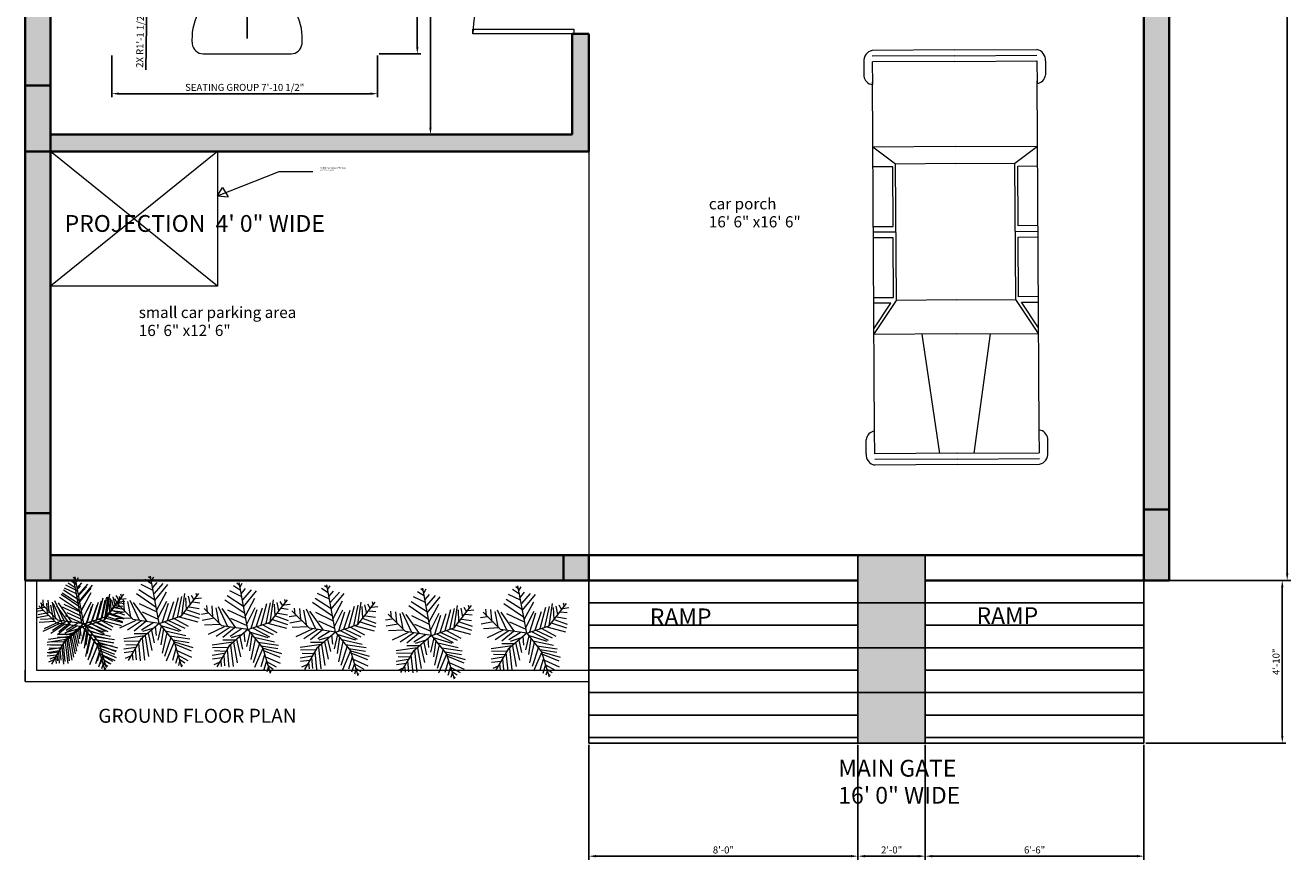
# Model space of a CAD drawing. Units: inches. Extents: x 2369 to 4208, y 1650 to 4492.
# Tile 1 of 6: x 2369 to 2820, y 1650 to 1948. Entities that reach past the tile are written whole.
import ezdxf

# ---------------------------------------------------------------- set-up
doc = ezdxf.new("R2010")
doc.units = ezdxf.units.IN
for name, color, linetype, lineweight in [('A-ANNO-DIMS', 2, 'Continuous', 13), ('A-ANNO-TEXT', 7, 'Continuous', 18), ('A-AREA-IDEN', 7, 'Continuous', 18), ('A-COLS', 7, 'Continuous', 35), ('A-COLS-PATT', 7, 'Continuous', 13), ('A-DOOR', 4, 'Continuous', 18), ('A-FLOR-PARK', 7, 'Continuous', 18), ('A-FLOR-RAMP', 7, 'Continuous', 25), ('A-FLOR-RAMP-PATT', 252, 'Continuous', 13), ('A-FURN', 8, 'Continuous', 18), ('A-FURN-VEHI', 8, 'Continuous', 13), ('A-WALL', 7, 'Continuous', 35), ('A-WALL-PATT', 252, 'Continuous', 13), ('L-PLNT-BEDS', 3, 'Continuous', 18), ('L-PLNT-TREE', 3, 'Continuous', 13), ('P-EQPM-TANK', 7, 'Continuous', 18)]:
    doc.layers.add(name, color=color, linetype=linetype, lineweight=lineweight)
doc.styles.get("Standard").update_dxf_attribs({"font": 'arial.ttf'})
doc.dimstyles.new('Copy of ISO-25', dxfattribs={"dimtxt": 2.5, "dimasz": 2.5, "dimexe": 1.25, "dimexo": 0.625, "dimtad": 1, "dimdec": 1, "dimlunit": 4, "dimtxsty": 'Standard', "dimcen": 2.5, "dimadec": 0, "dimazin": 0, "dimtfac": 1, "dimtdec": 1, "dimtmove": 0, "dimatfit": 3, "dimfxl": 1, "dimarcsym": 0})

# ---------------------------------------------------------------- blocks, each defined once
blk = doc.blocks.new('*U4')
for p, q in [((-40, 0), (-40, 6)), ((0, 0), (0, 6))]:
    blk.add_line(p, q)
blk.add_lwpolyline([(0, 0), (0, -40), (-1.75, -40), (-1.75, 0)], close=True)
blk.add_arc((0, 0), 40, 180, 270)
blk = doc.blocks.new('*D8')
at = {"layer": 'A-ANNO-DIMS', "color": 0, "lineweight": -2, "transparency": 16777216}
for p, q in [((2777.53, 2469.98), (2820.25, 2469.98)), ((2819, 2467.48), (2819, 1752.48)), ((2777.53, 1749.98), (2820.25, 1749.98))]:
    blk.add_line(p, q, dxfattribs=at)
at = {"layer": 'A-ANNO-DIMS', "color": 0, "transparency": 16777216}
for points in [[(2818.58, 2467.48), (2819.41, 2467.48), (2819, 2469.98)], [(2818.58, 1752.48), (2819.41, 1752.48), (2819, 1749.98)]]:
    blk.add_solid(points, dxfattribs=at)
at = {"layer": 'Defpoints', "color": 0, "transparency": 16777216}
for p in [(2776.9, 2469.98), (2776.9, 1749.98), (2819, 1749.98)]:
    blk.add_point(p, dxfattribs=at)
at = {"layer": 'A-ANNO-DIMS', "color": 0, "transparency": 16777216, "insert": (2817.1, 2109.98), "char_height": 2.5, "attachment_point": 5, "rotation": 90}
blk.add_mtext("60'", dxfattribs=at)
blk = doc.blocks.new('*D30')
at = {"layer": 'A-ANNO-DIMS', "color": 0, "lineweight": -2, "transparency": 16777216}
for p, q in [((2563.28, 2052.98), (2512.16, 2052.98)), ((2513.41, 2050.48), (2513.41, 1911.48)), ((2563.28, 1908.98), (2512.16, 1908.98))]:
    blk.add_line(p, q, dxfattribs=at)
at = {"layer": 'A-ANNO-DIMS', "color": 0, "transparency": 16777216}
for points in [[(2512.99, 2050.48), (2513.82, 2050.48), (2513.41, 2052.98)], [(2512.99, 1911.48), (2513.82, 1911.48), (2513.41, 1908.98)]]:
    blk.add_solid(points, dxfattribs=at)
at = {"layer": 'Defpoints', "color": 0, "transparency": 16777216}
for p in [(2563.9, 2052.98), (2513.41, 1908.98), (2563.9, 1908.98)]:
    blk.add_point(p, dxfattribs=at)
at = {"layer": 'A-ANNO-DIMS', "color": 0, "transparency": 16777216, "insert": (2511.53, 1980.98), "char_height": 2.5, "attachment_point": 5, "rotation": 90}
blk.add_mtext("12'", dxfattribs=at)
blk = doc.blocks.new('*U34')
for p, q in [((-7.288, 39.707), (-21.778, 46.673)), ((-8.737, 47.138), (-17.069, 52.711)), ((-10.186, 53.64), (-13.084, 55.962)), ((0, 0), (-10.5, 57)), ((-9.099, 51.782), (-6.563, 55.962)), ((-7.65, 43.423), (-2.578, 49.46)), ((-5.839, 35.992), (4.667, 48.067)), ((-5.114, 27.632), (10.463, 46.673)), ((-3.665, 19.273), (-27.574, 35.527)), ((-5.114, 28.097), (-24.676, 40.636)), ((-2.941, 16.486), (8.652, 37.85)), ((16.259, 5.805), (23.142, 31.348)), ((22.055, 7.198), (27.489, 32.277)), ((27, 9), (48, 36)), ((27.127, 9.056), (31.112, 35.992)), ((31.836, 30.883), (32.561, 16.486)), ((35.096, 32.741), (37.27, 22.524)), ((38.719, 34.134), (41.979, 28.561)), ((43.791, 29.954), (51.036, 30.883)), ((44.153, 36.456), (45.239, 32.741)), ((-47.498, 19.737), (-55.83, 18.344)), ((-31.5, 4.5), (-52.5, 25.5)), ((-48.585, 21.131), (-49.309, 29.026)), ((-43.513, 28.561), (-42.427, 15.558)), ((-38.442, 26.239), (-34.819, 7.663)), ((-35.544, 28.097), (-24.314, 3.947)), ((-14.533, 2.09), (-30.834, 25.31)), ((-24.314, 23.917), (-2.941, 13.7)), ((-1.129, 6.734), (9.014, 26.704)), ((3.942, 1.625), (11.187, 24.381)), ((10.101, 3.483), (17.708, 26.239)), ((33.285, 16.486), (48.862, 10.913)), ((36.183, 19.737), (48.137, 17.88)), ((40.53, 25.775), (48.862, 24.846)), ((-40.615, 13.7), (-55.105, 10.913)), ((-33.37, 6.269), (-52.207, 5.34)), ((-28.299, 3.483), (-47.86, -5.805)), ((-21.416, 3.018), (-38.079, -8.128)), ((0, 0), (-31.5, 4.5)), ((-15.982, 2.09), (-30.11, -9.521)), ((0, 0), (-22.5, -19.5)), ((-6.563, 1.161), (-21.416, -8.128)), ((-20.691, 13.7), (-1.129, 4.876)), ((0, 0), (27, 9)), ((0, 0), (18, -22.5)), ((6.478, 1.625), (26.04, -8.592)), ((11.187, 3.483), (30.749, -5.805)), ((18.07, 5.805), (35.096, -3.483)), ((24.229, 7.663), (46.688, 1.625)), ((29.662, 12.307), (48.137, 6.269)), ((-17.431, -15.094), (-42.789, -18.809)), ((-15.257, -12.772), (-30.11, -12.772)), ((-6.563, -5.805), (-19.967, -9.985)), ((-17.069, -15.094), (-12.721, -40.172)), ((-13.446, -11.378), (-8.737, -32.741)), ((-9.461, -8.592), (-6.201, -23.453)), ((-4.752, -3.483), (-3.665, -14.629)), ((2.493, -3.019), (-1.491, -20.202)), ((1.769, -2.555), (24.229, -9.521)), ((5.029, -6.27), (2.131, -25.775)), ((9.014, -11.378), (3.58, -35.992)), ((7.565, -9.056), (32.198, -14.629)), ((12.274, -15.094), (36.907, -18.809)), ((-28.299, -29.026), (-42.789, -31.348)), ((-24.314, -21.596), (-42.427, -22.06)), ((-26.849, -26.24), (-40.253, -25.775)), ((-22.5, -19.5), (-37.5, -45)), ((-25.038, -23.918), (-22.865, -45.281)), ((-20.691, -18.345), (-17.793, -44.352)), ((14.085, -16.951), (6.478, -40.172)), ((18.07, -22.524), (8.289, -45.745)), ((20.244, -30.419), (15.897, -44.816)), ((16.259, -19.738), (36.183, -22.989)), ((18, -22.5), (27, -52.5)), ((18.433, -22.524), (40.53, -29.026)), ((19.157, -25.311), (38.719, -33.206)), ((-30.834, -34.135), (-42.427, -35.528)), ((-34.457, -39.708), (-40.978, -42.494)), ((-32.646, -36.921), (-31.921, -44.352)), ((-29.023, -30.884), (-27.936, -43.887)), ((22.78, -37.85), (19.519, -48.532)), ((21.331, -32.741), (39.081, -40.636)), ((22.78, -38.314), (34.372, -44.816)), ((24.591, -45.745), (23.142, -50.854)), ((24.591, -43.423), (30.749, -47.603)), ((26.764, -49.925), (28.213, -50.854))]:
    blk.add_line(p, q)
blk = doc.blocks.new('*U36')
for p, q in [((138, 1075), (308, 1075)), ((4818, 1075), (4649, 1075)), ((3, -10), (3, 974)), ((70, -10), (70, 973)), ((138, 973), (410, 973)), ((138, -10), (138, 971)), ((410, 973), (4581, 973)), ((1563, -10), (1563, 973)), ((1563, 973), (1969, 702)), ((1630, 973), (1936, 769)), ((1936, 769), (1936, 973)), ((2003, 973), (2003, 736)), ((2716, 736), (2716, 973)), ((2783, 702), (2783, 973)), ((2851, 973), (2851, 736)), ((3563, 736), (3563, 973)), ((3597, 702), (3801, 973)), ((3801, -10), (3801, 973)), ((4818, 973), (4547, 973)), ((4818, -10), (4818, 971)), ((4886, -10), (4886, 973)), ((4954, -10), (4954, 974)), ((1969, 702), (3597, 702)), ((1969, -10), (1969, 702)), ((2003, 736), (2716, 736)), ((2851, 736), (3563, 736)), ((3597, -10), (3597, 702)), ((138, 193), (1563, 396)), ((3, -11), (3, -995)), ((70, -10), (70, -994)), ((138, -11), (138, -992)), ((1563, -10), (1563, -994)), ((1969, -10), (1969, -723)), ((3597, -10), (3597, -723)), ((3801, -10), (3801, -994)), ((4818, -11), (4818, -992)), ((4886, -10), (4886, -994)), ((4954, -11), (4954, -995)), ((138, -214), (1563, -417)), ((1563, -994), (1969, -723)), ((1969, -723), (3597, -723)), ((2783, -723), (2783, -994)), ((3597, -723), (3801, -994)), ((1630, -994), (1936, -790)), ((1936, -790), (1936, -994)), ((2003, -994), (2003, -757)), ((2003, -757), (2716, -757)), ((2716, -757), (2716, -994)), ((2851, -757), (3563, -757)), ((2851, -994), (2851, -757)), ((3563, -757), (3563, -994)), ((138, -994), (410, -994)), ((410, -994), (4581, -994)), ((4818, -994), (4547, -994)), ((138, -1096), (308, -1096)), ((4818, -1096), (4649, -1096))]:
    blk.add_line(p, q)
for centre, radius, start, end in [((128, 946), 129, 85.6455, 168.0943), ((291, 956), 120, 8.1301, 81.87), ((4665, 956), 120, 98.13, 171.8699), ((4828, 946), 129, 11.9057, 94.3545), ((128, -967), 129, 191.9057, 274.3545), ((291, -977), 120, 278.13, 351.8699), ((4665, -977), 120, 188.1301, 261.87), ((4828, -967), 129, 265.6455, 348.0943)]:
    blk.add_arc(centre, radius, start, end)
blk = doc.blocks.new('A$C22FC404C')
for p, q in [((1200, 1302), (1200, 1942)), ((809, 1143), (363, 1602)), ((1594, 1139), (2045, 1594)), ((0, 760), (640, 751)), ((2400, 731), (1760, 735)), ((827, 0), (1623, 0))]:
    blk.add_line(p, q)
for centre, radius, start, end in [((1200, 742), 1200, 359.499, 179.1174), ((1200, 742), 1040, 359.4096, 179.1174), ((1200, 742), 560, 359.3286, 179.1174), ((323, 870), 341, 199.1309, 339.1039), ((2082, 839), 341, 200.8961, 340.8691), ((1225, 139), 500, 354.3583, 185.6417), ((827, 100), 100, 185.6417, 270), ((1623, 100), 100, 270, 354.3583)]:
    blk.add_arc(centre, radius, start, end)
blk = doc.blocks.new('*D55')
at = {"layer": 'A-ANNO-DIMS', "color": 0, "lineweight": -2, "transparency": 16777216}
for p, q in [((2399.8, 1937.17), (2399.8, 1922.34)), ((2494.51, 1937.17), (2494.51, 1922.34)), ((2402.3, 1923.59), (2492.01, 1923.59))]:
    blk.add_line(p, q, dxfattribs=at)
at = {"layer": 'A-ANNO-DIMS', "color": 0, "transparency": 16777216}
for points in [[(2402.3, 1924.01), (2402.3, 1923.18), (2399.8, 1923.59)], [(2492.01, 1924.01), (2492.01, 1923.18), (2494.51, 1923.59)]]:
    blk.add_solid(points, dxfattribs=at)
at = {"layer": 'Defpoints', "color": 0, "transparency": 16777216}
for p in [(2399.8, 1937.8), (2494.51, 1937.8), (2494.51, 1923.59)]:
    blk.add_point(p, dxfattribs=at)
at = {"layer": 'A-ANNO-DIMS', "color": 0, "transparency": 16777216, "insert": (2447.15, 1925.51), "char_height": 2.5, "attachment_point": 5}
blk.add_mtext('SEATING GROUP 7\'-10 1/2"', dxfattribs=at)
blk = doc.blocks.new('*D56')
at = {"layer": 'A-ANNO-DIMS', "color": 0, "lineweight": -2, "transparency": 16777216}
for p, q in [((2495.13, 2014.56), (2509.96, 2014.56)), ((2508.71, 1940.3), (2508.71, 2012.06)), ((2495.13, 1937.8), (2509.96, 1937.8))]:
    blk.add_line(p, q, dxfattribs=at)
at = {"layer": 'A-ANNO-DIMS', "color": 0, "transparency": 16777216}
for points in [[(2508.3, 2012.06), (2509.13, 2012.06), (2508.71, 2014.56)], [(2508.3, 1940.3), (2509.13, 1940.3), (2508.71, 1937.8)]]:
    blk.add_solid(points, dxfattribs=at)
at = {"layer": 'Defpoints', "color": 0, "transparency": 16777216}
for p in [(2494.51, 2014.56), (2508.71, 2014.56), (2494.51, 1937.8)]:
    blk.add_point(p, dxfattribs=at)
at = {"layer": 'A-ANNO-DIMS', "color": 0, "transparency": 16777216, "insert": (2506.81, 1976.18), "char_height": 2.5, "attachment_point": 5, "rotation": 90}
blk.add_mtext('6\'-5"', dxfattribs=at)
blk = doc.blocks.new('*D57')
at = {"layer": 'A-ANNO-DIMS', "color": 0, "lineweight": -2, "transparency": 16777216}
for p, q in [((2768.53, 1749.98), (2818.5, 1749.98)), ((2817.25, 1694.48), (2817.25, 1747.48)), ((2768.53, 1691.98), (2818.5, 1691.98))]:
    blk.add_line(p, q, dxfattribs=at)
at = {"layer": 'A-ANNO-DIMS', "color": 0, "transparency": 16777216}
for points in [[(2816.83, 1747.48), (2817.67, 1747.48), (2817.25, 1749.98)], [(2816.83, 1694.48), (2817.67, 1694.48), (2817.25, 1691.98)]]:
    blk.add_solid(points, dxfattribs=at)
at = {"layer": 'Defpoints', "color": 0, "transparency": 16777216}
for p in [(2767.9, 1749.98), (2817.25, 1749.98), (2767.9, 1691.98)]:
    blk.add_point(p, dxfattribs=at)
at = {"layer": 'A-ANNO-DIMS', "color": 0, "transparency": 16777216, "insert": (2815.35, 1720.98), "char_height": 2.5, "attachment_point": 5, "rotation": 90}
blk.add_mtext('4\'-10"', dxfattribs=at)
blk = doc.blocks.new('*D58')
at = {"layer": 'A-ANNO-DIMS', "color": 0, "lineweight": -2, "transparency": 16777216}
for p, q in [((2569.9, 1691.35), (2569.9, 1650.38)), ((2665.9, 1691.35), (2665.9, 1650.38)), ((2572.4, 1651.63), (2663.4, 1651.63))]:
    blk.add_line(p, q, dxfattribs=at)
at = {"layer": 'A-ANNO-DIMS', "color": 0, "transparency": 16777216}
for points in [[(2572.4, 1652.05), (2572.4, 1651.21), (2569.9, 1651.63)], [(2663.4, 1652.05), (2663.4, 1651.21), (2665.9, 1651.63)]]:
    blk.add_solid(points, dxfattribs=at)
at = {"layer": 'Defpoints', "color": 0, "transparency": 16777216}
for p in [(2569.9, 1691.98), (2665.9, 1691.98), (2665.9, 1651.63)]:
    blk.add_point(p, dxfattribs=at)
at = {"layer": 'A-ANNO-DIMS', "color": 0, "transparency": 16777216, "insert": (2617.9, 1653.53), "char_height": 2.5, "attachment_point": 5}
blk.add_mtext('8\'-0"', dxfattribs=at)
blk = doc.blocks.new('*D59')
at = {"layer": 'A-ANNO-DIMS', "color": 0, "lineweight": -2, "transparency": 16777216}
for p, q in [((2665.9, 1691.35), (2665.9, 1650.38)), ((2689.9, 1691.35), (2689.9, 1650.38)), ((2668.4, 1651.63), (2687.4, 1651.63))]:
    blk.add_line(p, q, dxfattribs=at)
at = {"layer": 'A-ANNO-DIMS', "color": 0, "transparency": 16777216}
for points in [[(2668.4, 1652.05), (2668.4, 1651.21), (2665.9, 1651.63)], [(2687.4, 1652.05), (2687.4, 1651.21), (2689.9, 1651.63)]]:
    blk.add_solid(points, dxfattribs=at)
at = {"layer": 'Defpoints', "color": 0, "transparency": 16777216}
for p in [(2665.9, 1691.98), (2689.9, 1691.98), (2689.9, 1651.63)]:
    blk.add_point(p, dxfattribs=at)
at = {"layer": 'A-ANNO-DIMS', "color": 0, "transparency": 16777216, "insert": (2677.9, 1653.53), "char_height": 2.5, "attachment_point": 5}
blk.add_mtext('2\'-0"', dxfattribs=at)
blk = doc.blocks.new('*D60')
at = {"layer": 'A-ANNO-DIMS', "color": 0, "lineweight": -2, "transparency": 16777216}
for p, q in [((2689.9, 1691.35), (2689.9, 1650.38)), ((2767.9, 1691.35), (2767.9, 1650.38)), ((2692.4, 1651.63), (2765.4, 1651.63))]:
    blk.add_line(p, q, dxfattribs=at)
at = {"layer": 'A-ANNO-DIMS', "color": 0, "transparency": 16777216}
for points in [[(2692.4, 1652.05), (2692.4, 1651.21), (2689.9, 1651.63)], [(2765.4, 1652.05), (2765.4, 1651.21), (2767.9, 1651.63)]]:
    blk.add_solid(points, dxfattribs=at)
at = {"layer": 'Defpoints', "color": 0, "transparency": 16777216}
for p in [(2689.9, 1691.98), (2767.9, 1691.98), (2767.9, 1651.63)]:
    blk.add_point(p, dxfattribs=at)
at = {"layer": 'A-ANNO-DIMS', "color": 0, "transparency": 16777216, "insert": (2728.9, 1653.53), "char_height": 2.5, "attachment_point": 5}
blk.add_mtext('6\'-6"', dxfattribs=at)
blk = doc.blocks.new('*D71')
at = {"layer": 'A-ANNO-DIMS', "color": 0, "lineweight": -2, "transparency": 16777216}
for p, q in [((2448.04, 1984.08), (2448.04, 1965.47)), ((2448.04, 1943.28), (2448.04, 1962.97))]:
    blk.add_line(p, q, dxfattribs=at)
at = {"layer": 'A-ANNO-DIMS', "color": 0, "transparency": 16777216}
blk.add_solid([(2447.62, 1965.47), (2448.46, 1965.47), (2448.04, 1962.97)], dxfattribs=at)
at = {"layer": 'Defpoints', "color": 0, "transparency": 16777216}
for p in [(2448.04, 1962.97), (2448.04, 1943.28)]:
    blk.add_point(p, dxfattribs=at)
at = {"layer": 'A-ANNO-DIMS', "color": 0, "transparency": 16777216, "insert": (2446.12, 1976.03), "char_height": 2.5, "attachment_point": 5, "rotation": 89.9986}
blk.add_mtext('R1\'-7 1/2"', dxfattribs=at)
blk = doc.blocks.new('*D72')
at = {"layer": 'A-ANNO-DIMS', "color": 0, "lineweight": -2, "transparency": 16777216}
for p, q in [((2412.52, 1972.03), (2412.31, 1958.63)), ((2411.91, 1932.1), (2412.28, 1956.13))]:
    blk.add_line(p, q, dxfattribs=at)
at = {"layer": 'A-ANNO-DIMS', "color": 0, "transparency": 16777216}
blk.add_solid([(2411.86, 1956.13), (2412.69, 1956.12), (2412.31, 1958.63)], dxfattribs=at)
at = {"layer": 'Defpoints', "color": 0, "transparency": 16777216}
for p in [(2412.52, 1972.03), (2412.31, 1958.63)]:
    blk.add_point(p, dxfattribs=at)
at = {"layer": 'A-ANNO-DIMS', "color": 0, "transparency": 16777216, "insert": (2410.16, 1942.89), "char_height": 2.5, "attachment_point": 5, "rotation": 89.1191}
blk.add_mtext('2X R1\'-1 1/2"', dxfattribs=at)

msp = doc.modelspace()

# ---------------------------------------------------------------- hatches: boundary and pattern name
at = {"layer": 'A-COLS-PATT'}
h = msp.add_hatch(color=256, dxfattribs=at)
h.dxf.hatch_style = 1
h.paths.add_polyline_path([(2377.9, 2254.21), (2368.9, 2254.21), (2368.9, 2226.98), (2377.9, 2226.98)])
h.paths.add_polyline_path([(2551.9, 2400.98), (2545.9, 2400.98), (2525.15, 2400.98), (2525.15, 2394.98), (2545.9, 2395.12), (2551.9, 2395.12)])
h.paths.add_polyline_path([(2637.99, 2400.98), (2599.9, 2400.98), (2599.9, 2394.98), (2605.9, 2394.98), (2637.99, 2394.98)])
h.paths.add_polyline_path([(2623.27, 2232.98), (2599.9, 2232.98), (2599.9, 2226.98), (2623.27, 2226.98)])
h.paths.add_polyline_path([(2551.9, 2232.98), (2528.53, 2232.98), (2528.53, 2226.98), (2551.9, 2226.98)])
h.paths.add_polyline_path([(2731.9, 2232.98), (2713.81, 2232.98), (2713.81, 2226.98), (2731.9, 2226.98)])
h.paths.add_polyline_path([(2776.9, 2250.53), (2767.9, 2250.53), (2767.9, 2232.98), (2767.9, 2226.98), (2776.9, 2226.98)])
h.paths.add_polyline_path([(2776.9, 2078.3), (2767.9, 2078.3), (2767.9, 2058.98), (2767.9, 2052.98), (2776.9, 2052.98)])
h.paths.add_polyline_path([(2731.9, 2058.98), (2725.9, 2058.98), (2713.81, 2058.98), (2713.81, 2052.98), (2731.9, 2052.98)])
h.paths.add_polyline_path([(2776.9, 1973.96), (2767.9, 1973.96), (2767.9, 1956.98), (2767.9, 1950.98), (2776.9, 1950.98)])
h.paths.add_polyline_path([(2776.9, 1775.33), (2767.9, 1775.33), (2767.9, 1758.98), (2767.9, 1749.98), (2776.9, 1749.98)])
h.paths.add_polyline_path([(2569.9, 1758.98), (2560.9, 1758.98), (2560.9, 1749.98), (2569.9, 1749.98)])
h.paths.add_polyline_path([(2377.9, 1774.03), (2368.9, 1774.03), (2368.9, 1749.98), (2372.9, 1749.98), (2377.9, 1749.98)])
h.paths.add_polyline_path([(2377.9, 1926.53), (2368.9, 1926.53), (2368.9, 1902.98), (2377.9, 1902.98)])
h.paths.add_polyline_path([(2377.9, 2079.34), (2368.9, 2079.34), (2368.9, 2052.98), (2377.9, 2052.98), (2377.9, 2057.9)])
at = {"layer": 'A-FLOR-RAMP-PATT'}
h = msp.add_hatch(color=256, dxfattribs=at)
h.dxf.hatch_style = 1
h.paths.add_polyline_path([(2689.9, 1758.98), (2665.9, 1758.98), (2665.9, 1741.98), (2689.9, 1741.98)])
h.paths.add_polyline_path([(2689.9, 1741.98), (2665.9, 1741.98), (2665.9, 1725.98), (2689.9, 1725.98)])
h.paths.add_polyline_path([(2689.9, 1725.98), (2665.9, 1725.98), (2665.9, 1709.98), (2689.9, 1709.98)])
h.paths.add_polyline_path([(2689.9, 1709.98), (2665.9, 1709.98), (2665.9, 1691.98), (2689.9, 1691.98)])
at = {"layer": 'A-WALL-PATT'}
h = msp.add_hatch(color=256, dxfattribs=at)
h.dxf.hatch_style = 1
h.paths.add_polyline_path([(2377.9, 2052.98), (2368.9, 2052.98), (2368.9, 1926.53), (2377.9, 1926.53)])
h.paths.add_polyline_path([(2377.9, 2226.98), (2368.9, 2226.98), (2368.9, 2079.34), (2377.9, 2079.34)])
h.paths.add_polyline_path([(2377.9, 2394.98), (2377.9, 2460.98), (2767.9, 2460.98), (2767.9, 2250.53), (2776.9, 2250.53), (2776.9, 2469.98), (2368.9, 2469.98), (2368.9, 2254.21), (2377.9, 2254.21)])
h.paths.add_polyline_path([(2776.9, 2226.98), (2767.9, 2226.98), (2767.9, 2078.3), (2776.9, 2078.3)])
h.paths.add_polyline_path([(2776.9, 2052.98), (2767.9, 2052.98), (2767.9, 1973.96), (2776.9, 1973.96)])
h.paths.add_polyline_path([(2776.9, 1950.98), (2767.9, 1950.98), (2767.9, 1775.33), (2776.9, 1775.33)])
h.paths.add_polyline_path([(2560.9, 1758.98), (2377.9, 1758.98), (2377.9, 1749.98), (2386.24, 1749.98), (2386.07, 1750.89), (2387.22, 1749.98), (2560.9, 1749.98)])
h.paths.add_polyline_path([(2377.9, 1902.98), (2368.9, 1902.98), (2368.9, 1774.03), (2377.9, 1774.03)])
h.paths.add_polyline_path([(2569.9, 1908.98), (2569.9, 1944.98), (2563.9, 1944.98), (2563.9, 1908.98), (2377.9, 1908.98), (2377.9, 1902.98), (2569.9, 1902.98)])
h.paths.add_polyline_path([(2523.29, 2058.98), (2411, 2058.98), (2411, 2052.98), (2523.29, 2052.98)])
h.paths.add_polyline_path([(2569.9, 2052.98), (2641.9, 2052.98), (2713.81, 2052.98), (2713.81, 2058.98), (2559.29, 2058.98), (2559.29, 2052.98), (2563.9, 2052.98), (2563.9, 1980.98), (2569.9, 1980.98), (2569.9, 1992.98)])
h.paths.add_polyline_path([(2528.53, 2232.98), (2510.56, 2232.98), (2377.9, 2232.98), (2377.9, 2226.98), (2528.53, 2226.98)])
h.paths.add_polyline_path([(2713.81, 2232.98), (2623.27, 2232.98), (2623.27, 2226.98), (2713.81, 2226.98)])
h.paths.add_polyline_path([(2647.9, 2008.36), (2642.51, 2008.36), (2641.9, 2008.36), (2641.9, 1956.98), (2641.9, 1950.98), (2767.9, 1950.98), (2767.9, 1956.98), (2647.9, 1956.98)])
h.paths.add_polyline_path([(2551.9, 2395.12), (2545.9, 2395.12), (2545.9, 2268.98), (2551.9, 2268.98)], flags=17)
h.paths.add_polyline_path([(2551.9, 2460.98), (2545.9, 2460.98), (2545.9, 2400.98), (2551.9, 2400.98)], flags=17)
h.paths.add_polyline_path([(2605.9, 2460.98), (2599.9, 2460.98), (2599.9, 2400.98), (2605.9, 2400.98)], flags=17)
h.paths.add_polyline_path([(2767.9, 2400.98), (2637.99, 2400.98), (2637.99, 2394.98), (2767.9, 2394.98)], flags=17)
h.paths.add_polyline_path([(2605.9, 2394.98), (2599.9, 2394.98), (2599.9, 2394.42), (2599.9, 2268.98), (2605.9, 2268.98)], flags=17)
h.paths.add_polyline_path([(2525.15, 2400.98), (2377.9, 2400.98), (2377.9, 2394.98), (2525.15, 2394.98)], flags=17)
h.paths.add_polyline_path([(2449.9, 2412.98), (2444.51, 2412.98), (2443.9, 2412.98), (2443.9, 2400.98), (2449.9, 2400.98)], flags=17)
h.paths.add_polyline_path([(2449.9, 2460.98), (2443.9, 2460.98), (2443.9, 2448.98), (2449.9, 2448.98)], flags=17)
h.paths.add_polyline_path([(2731.9, 2106.98), (2725.9, 2106.98), (2725.9, 2058.98), (2731.9, 2058.98)])

# ---------------------------------------------------------------- linework, layer by layer
at = {"layer": 'A-ANNO-TEXT'}
for p, q in [((2437.49, 1887.16), (2459.47, 1895.88)), ((2459.47, 1895.88), (2471.48, 1895.88)), ((2437.49, 1887.16), (2439.18, 1890.11)), ((2437.49, 1887.16), (2441.31, 1886.78)), ((2439.18, 1890.11), (2441.31, 1886.78))]:
    msp.add_line(p, q, dxfattribs=at)
at = {"layer": 'A-COLS'}
for p, q in [((2368.9, 1902.98), (2368.9, 1926.53)), ((2368.9, 1926.53), (2377.9, 1926.53)), ((2377.9, 1902.98), (2368.9, 1902.98)), ((2368.9, 1749.98), (2368.9, 1774.03)), ((2368.9, 1774.03), (2377.9, 1774.03)), ((2377.9, 1774.03), (2377.9, 1749.98)), ((2776.9, 1775.33), (2767.9, 1775.33)), ((2776.9, 1749.98), (2776.9, 1775.33)), ((2569.9, 1758.98), (2560.9, 1758.98)), ((2560.9, 1758.98), (2560.9, 1749.98)), ((2569.9, 1758.98), (2569.9, 1749.98)), ((2569.9, 1749.98), (2569.9, 1758.98)), ((2767.9, 1758.98), (2767.9, 1749.98)), ((2372.9, 1749.98), (2368.9, 1749.98))]:
    msp.add_line(p, q, dxfattribs=at)
at = {"layer": 'A-FLOR-PARK'}
msp.add_line((2569.9, 1902.98), (2569.9, 1758.98), dxfattribs=at)
at = {"layer": 'A-FLOR-RAMP'}
for p, q in [((2665.9, 1691.98), (2665.9, 1758.98)), ((2665.9, 1758.98), (2689.9, 1758.98)), ((2689.9, 1758.98), (2689.9, 1691.98)), ((2569.9, 1749.98), (2569.9, 1691.98)), ((2569.9, 1749.98), (2569.9, 1741.98)), ((2767.9, 1691.98), (2767.9, 1749.98)), ((2569.9, 1741.98), (2665.9, 1741.98)), ((2665.9, 1741.98), (2689.9, 1741.98)), ((2689.9, 1741.98), (2767.9, 1741.98)), ((2689.9, 1741.98), (2689.9, 1725.98)), ((2767.9, 1741.98), (2767.9, 1733.98)), ((2569.9, 1733.98), (2569.9, 1725.98)), ((2665.9, 1733.98), (2569.9, 1733.98)), ((2767.9, 1733.98), (2689.9, 1733.98)), ((2569.9, 1725.98), (2665.9, 1725.98)), ((2689.9, 1725.98), (2665.9, 1725.98)), ((2665.9, 1725.98), (2665.9, 1709.98)), ((2689.9, 1725.98), (2767.9, 1725.98)), ((2767.9, 1725.98), (2767.9, 1717.98)), ((2569.9, 1717.98), (2569.9, 1709.98)), ((2665.9, 1717.98), (2569.9, 1717.98)), ((2767.9, 1717.98), (2689.9, 1717.98)), ((2569.9, 1709.98), (2665.9, 1709.98)), ((2665.9, 1709.98), (2689.9, 1709.98)), ((2689.9, 1709.98), (2767.9, 1709.98)), ((2689.9, 1709.98), (2689.9, 1691.98)), ((2767.9, 1709.98), (2767.9, 1701.98)), ((2569.9, 1701.98), (2569.9, 1693.98)), ((2665.9, 1701.98), (2569.9, 1701.98)), ((2767.9, 1701.98), (2689.9, 1701.98)), ((2569.9, 1693.98), (2665.9, 1693.98)), ((2689.9, 1693.98), (2767.9, 1693.98)), ((2767.9, 1693.98), (2767.9, 1691.98)), ((2569.9, 1691.98), (2665.9, 1691.98)), ((2665.9, 1691.98), (2569.9, 1691.98)), ((2689.9, 1691.98), (2665.9, 1691.98)), ((2767.9, 1691.98), (2689.9, 1691.98))]:
    msp.add_line(p, q, dxfattribs=at)
at = {"layer": 'A-WALL'}
for p, q in [((2377.9, 2052.98), (2377.9, 1908.98)), ((2563.9, 1908.98), (2563.9, 1944.98)), ((2569.9, 1944.98), (2563.9, 1944.98)), ((2569.9, 1944.98), (2569.9, 1908.98)), ((2377.9, 1908.98), (2563.9, 1908.98)), ((2569.9, 1908.98), (2569.9, 1902.98)), ((2569.9, 1902.98), (2377.9, 1902.98))]:
    msp.add_line(p, q, dxfattribs=at)
for points in [[(2368.9, 1749.98), (2368.9, 2469.98), (2776.9, 2469.98), (2776.9, 1749.98), (2689.9, 1749.98)], [(2767.9, 2052.98), (2767.9, 1758.98), (2377.9, 1758.98), (2377.9, 2460.98), (2767.9, 2460.98), (2767.9, 2232.98)], [(2665.9, 1749.98), (2372.9, 1749.98)]]:
    msp.add_lwpolyline(points, dxfattribs=at)
at = {"layer": 'L-PLNT-BEDS'}
for p, q in [((2368.9, 1749.98), (2368.9, 1713.98)), ((2372.9, 1749.98), (2372.9, 1717.98)), ((2368.9, 1713.98), (2368.9, 1717.98)), ((2372.9, 1717.98), (2569.9, 1717.98)), ((2368.9, 1713.98), (2569.9, 1713.98))]:
    msp.add_line(p, q, dxfattribs=at)
at = {"layer": 'P-EQPM-TANK'}
for p, q in [((2377.9, 1902.98), (2437.49, 1902.98)), ((2437.49, 1854.98), (2377.9, 1902.98)), ((2437.49, 1902.98), (2377.9, 1854.98)), ((2437.49, 1902.98), (2437.49, 1854.98)), ((2437.49, 1854.98), (2377.9, 1854.98))]:
    msp.add_line(p, q, dxfattribs=at)

# ---------------------------------------------------------------- block references
at = {"layer": 'A-DOOR', "xscale": 0.8987594980764617, "yscale": 0.8987594980764617, "zscale": 0.8987594980764617, "rotation": 270}
msp.add_blockref('*U4', (2564.51, 1944.98), dxfattribs=at)
at = {"layer": 'A-FURN', "xscale": 0.0393700787401575, "yscale": 0.0393700787401575, "zscale": 0.0393700787401575}
msp.add_blockref('A$C22FC404C', (2399.8, 1937.8), dxfattribs=at)
at = {"layer": 'A-FURN-VEHI', "xscale": 0.0298702624736708, "yscale": 0.0298702624736708, "zscale": 0.0298702624736708, "rotation": 90.35493414145904}
msp.add_blockref('*U36', (2700.95, 1791.2), dxfattribs=at)
at = {"layer": 'L-PLNT-TREE', "xscale": 0.2955086411556793, "yscale": 0.2955086411556793, "zscale": 0.2955086411556793}
for p in [(2389.8, 1734.47), (2416.66, 1734.68), (2389.29, 1733.44), (2448.25, 1732.44), (2479.54, 1731.57), (2513.84, 1730.39), (2547.74, 1731.17)]:
    msp.add_blockref('*U34', p, dxfattribs=at)

# ---------------------------------------------------------------- texts
at = {"layer": 'A-ANNO-TEXT'}
for s, height, p in [('3\' 0" X6\' 0" X4\' 0"', 0.4729, (2474.12, 1896.05)), ('UNDER  GROUND WATER TANK', 0.4729, (2474.12, 1896.81)), ('PROJECTION  4\' 0" WIDE', 6, (2382.94, 1874.3)), ('RAMP', 6, (2591.66, 1733.98)), ('RAMP', 6, (2708.19, 1734.42)), ('GROUND FLOOR PLAN', 5, (2394.94, 1699.21)), ('MAIN GATE', 6, (2658.88, 1680)), ('16\' 0" WIDE', 6, (2658.88, 1670.36))]:
    msp.add_text(s, height=height, dxfattribs=at).set_placement(p)
at = {"layer": 'A-AREA-IDEN'}
for s, p in [('car porch', (2612.71, 1882.33)), ('16\' 6" x16\' 6"', (2612.71, 1875.9)), ('small car parking area', (2409.37, 1843.58)), ('16\' 6" x12\' 6"', (2409.37, 1837.15))]:
    msp.add_text(s, height=4, dxfattribs=at).set_placement(p)

# ---------------------------------------------------------------- dimensions: what is measured, and where the dimension line sits
at = {"layer": 'A-ANNO-DIMS'}
for base, p1, p2, override, picture, middle in [((2819, 1749.98), (2776.9, 2469.98), (2776.9, 1749.98), {"dimclrd": 0, "dimclre": 0, "dimclrt": 0}, '*D8', (2817.1, 2109.98)), ((2513.41, 1908.98), (2563.9, 2052.98), (2563.9, 1908.98), {"dimclrd": 0, "dimclre": 0, "dimclrt": 0}, '*D30', (2511.53, 1980.98)), ((2508.71, 2014.56), (2494.51, 1937.8), (2494.51, 2014.56), {"dimdec": 1, "dimlfac": 1, "dimrnd": 0, "dimzin": 1, "dimdsep": 46, "dimlunit": 4, "dimfrac": 2}, '*D56', (2506.81, 1976.18)), ((2817.25, 1749.98), (2767.9, 1691.98), (2767.9, 1749.98), {"dimdec": 1, "dimlfac": 1, "dimrnd": 0, "dimzin": 1, "dimdsep": 46, "dimlunit": 4, "dimfrac": 2}, '*D57', (2815.35, 1720.98))]:
    dim = msp.add_linear_dim(base=base, p1=p1, p2=p2, angle=90, dimstyle='Copy of ISO-25', override=override, dxfattribs=at)
    dim.commit()
    dim.dimension.update_dxf_attribs({"geometry": picture, "text_midpoint": middle})
dim = msp.add_radius_dim(center=(2448.04, 1943.28), mpoint=(2448.04, 1962.97), dimstyle='Copy of ISO-25', override={"dimdec": 1, "dimlfac": 1, "dimrnd": 0, "dimzin": 1, "dimdsep": 46, "dimlunit": 4, "dimfrac": 2}, dxfattribs=at)
dim.commit()
dim.dimension.update_dxf_attribs({"geometry": '*D71', "text_midpoint": (2446.12, 1976.03)})
dim = msp.add_radius_dim(center=(2412.52, 1972.03), mpoint=(2412.31, 1958.63), text='2X <>', dimstyle='Copy of ISO-25', override={"dimdec": 1, "dimlfac": 1, "dimrnd": 0, "dimzin": 1, "dimdsep": 46, "dimlunit": 4, "dimfrac": 2}, dxfattribs=at)
dim.commit()
dim.dimension.update_dxf_attribs({"geometry": '*D72', "text_midpoint": (2410.16, 1942.89)})
dim = msp.add_linear_dim(base=(2494.51, 1923.59), p1=(2399.8, 1937.8), p2=(2494.51, 1937.8), text='SEATING GROUP <>', dimstyle='Copy of ISO-25', override={"dimdec": 1, "dimlfac": 1, "dimrnd": 0, "dimzin": 1, "dimdsep": 46, "dimlunit": 4, "dimfrac": 2}, dxfattribs=at)
dim.commit()
dim.dimension.update_dxf_attribs({"geometry": '*D55', "text_midpoint": (2447.15, 1925.51)})
for base, p1, p2, picture, middle in [((2665.9, 1651.63), (2569.9, 1691.98), (2665.9, 1691.98), '*D58', (2617.9, 1653.53)), ((2689.9, 1651.63), (2665.9, 1691.98), (2689.9, 1691.98), '*D59', (2677.9, 1653.53)), ((2767.9, 1651.63), (2689.9, 1691.98), (2767.9, 1691.98), '*D60', (2728.9, 1653.53))]:
    dim = msp.add_linear_dim(base=base, p1=p1, p2=p2, dimstyle='Copy of ISO-25', override={"dimdec": 1, "dimlfac": 1, "dimrnd": 0, "dimzin": 1, "dimdsep": 46, "dimlunit": 4, "dimfrac": 2}, dxfattribs=at)
    dim.commit()
    dim.dimension.update_dxf_attribs({"geometry": picture, "text_midpoint": middle})

doc.saveas('drawing.dxf')
